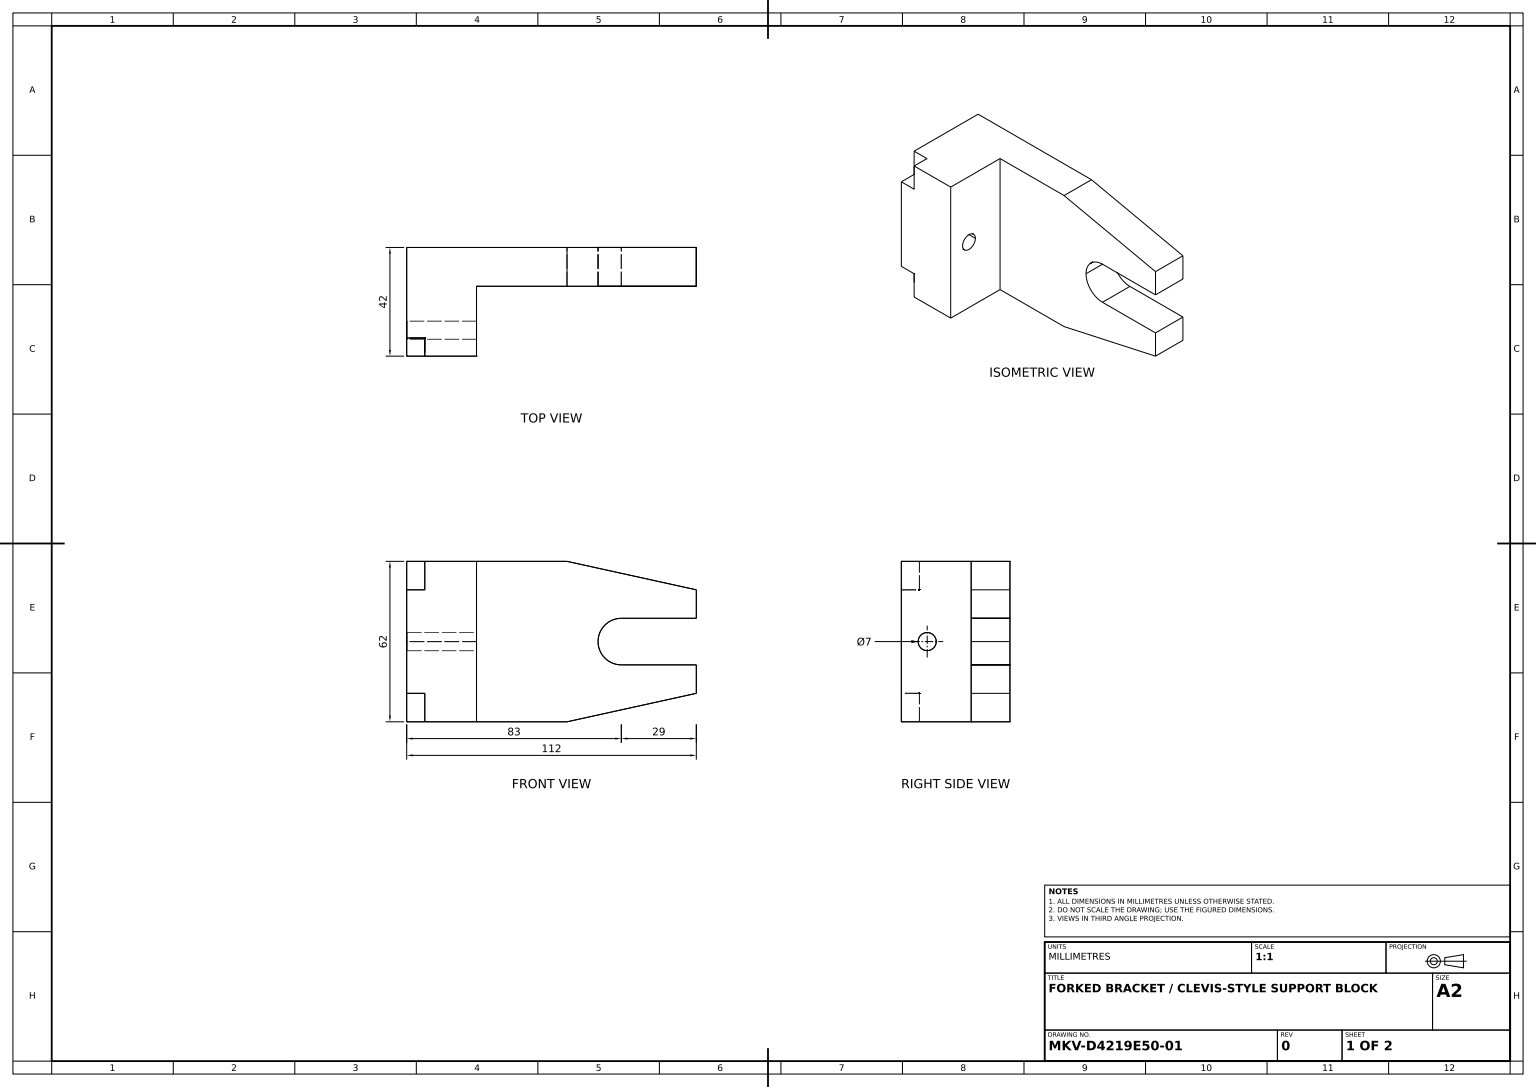
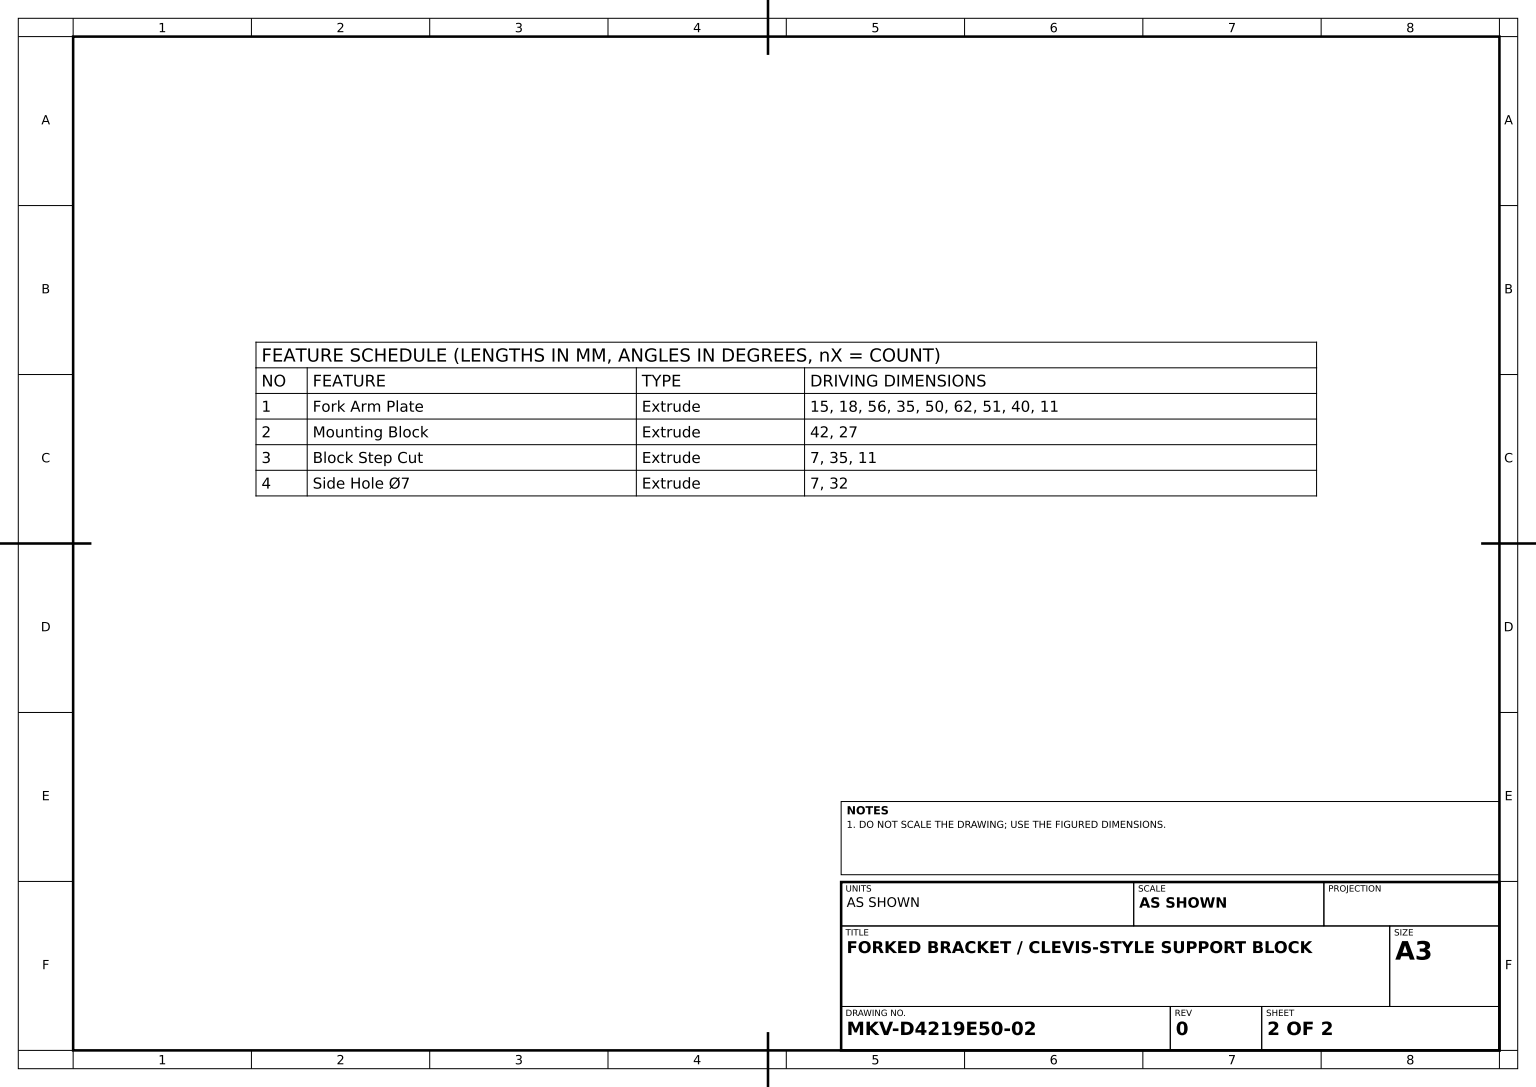
from build123d import *

# Parameters (mm, degrees)
FORK_ARM_PLATE_DEPTH    = 15
MOUNTING_BLOCK_SKETCH_W = 27
MOUNTING_BLOCK_SKETCH_H = 62
MOUNTING_BLOCK_DEPTH    = 42
BLOCK_STEP_CUT_SKETCH_W = 7
BLOCK_STEP_CUT_SKETCH_H = 11
BLOCK_STEP_CUT_DEPTH    = 7
SIDE_HOLE_7_SKETCH_R    = 3.5
SIDE_HOLE_7_DEPTH       = 135.729358345


with BuildPart() as part:
    # Fork Arm Profile Sketch → Fork Arm Plate (new body)
    with BuildSketch(Plane.XY):
        with BuildLine():
            ThreePointArc((56, 40), (47, 31), (56, 22))
            Line((56, 22), (85, 22))
            Line((85, 22), (85, 11))
            Line((85, 11), (35, 0))
            Line((35, 0), (0, 0))
            Line((0, 0), (0, 62))
            Line((0, 62), (35, 62))
            Line((35, 62), (85, 51))
            Line((85, 51), (85, 40))
            Line((85, 40), (56, 40))
        make_face()
    extrude(amount=FORK_ARM_PLATE_DEPTH)

    # Mounting Block Sketch → Mounting Block (add)
    with BuildSketch(Plane.XY):
        with Locations((-13.5, 31)):
            Rectangle(MOUNTING_BLOCK_SKETCH_W, MOUNTING_BLOCK_SKETCH_H)
    extrude(amount=MOUNTING_BLOCK_DEPTH)

    # Block Step Cut Sketch → Block Step Cut (cut)
    with BuildSketch(Plane.ZY.offset(27)):
        with Locations((38.5, 56.5)):
            Rectangle(BLOCK_STEP_CUT_SKETCH_W, BLOCK_STEP_CUT_SKETCH_H)
        with Locations((38.5, 5.5)):
            Rectangle(BLOCK_STEP_CUT_SKETCH_W, BLOCK_STEP_CUT_SKETCH_H)
    extrude(amount=-BLOCK_STEP_CUT_DEPTH, mode=Mode.SUBTRACT)

    # Side Hole Ø7 Sketch → Side Hole Ø7 (cut, through all)
    with BuildSketch(Plane.ZY.offset(27)):
        with Locations((32, 31)):
            Circle(SIDE_HOLE_7_SKETCH_R)
    extrude(amount=-SIDE_HOLE_7_DEPTH, mode=Mode.SUBTRACT)


solid = part.part
